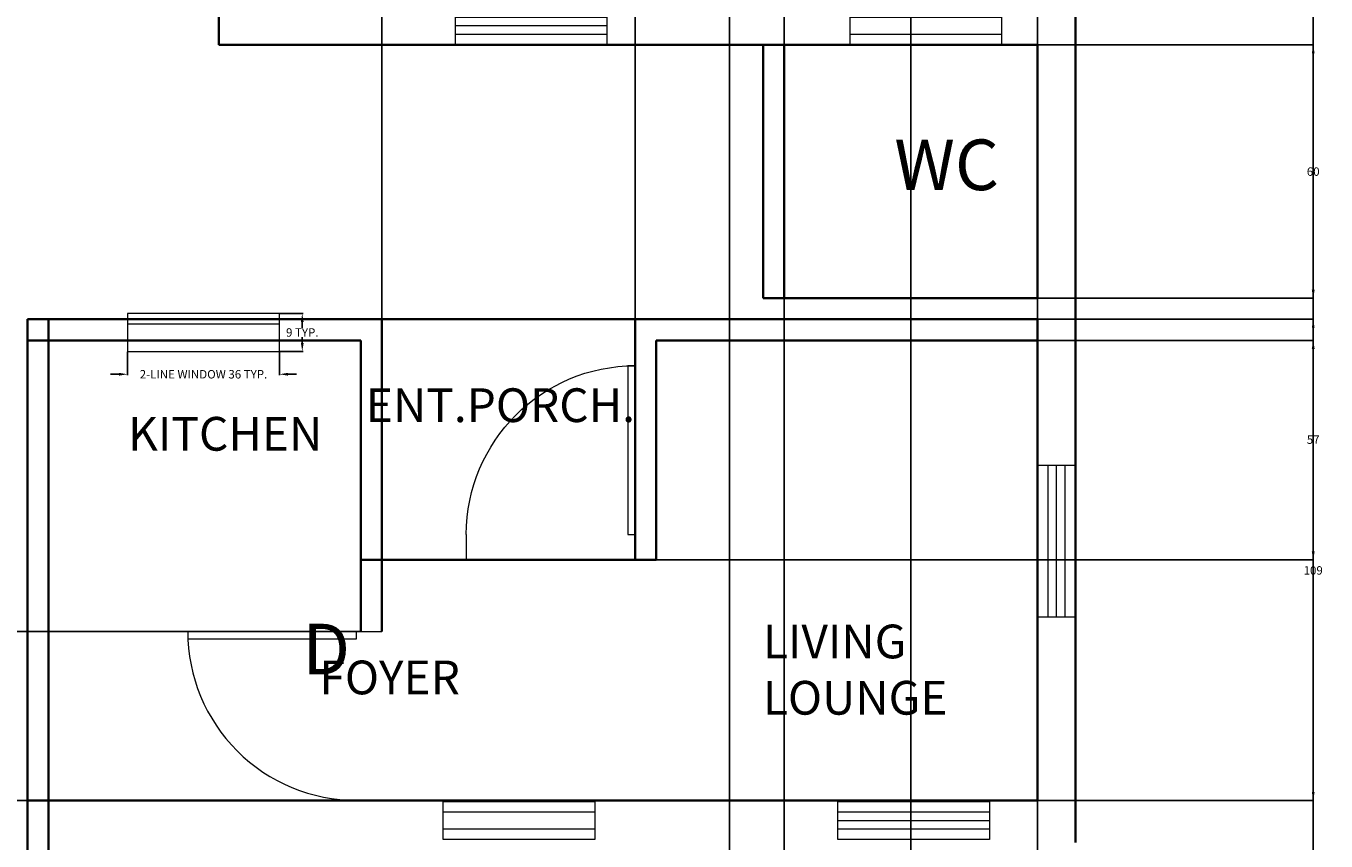
# Model space of a CAD drawing. Units: inches. Extents: x 190 to 836, y -241 to 999.
# Tile 4 of 9: x 528 to 836, y -8 to 185. Entities that reach past the tile are written whole.
import ezdxf

# ---------------------------------------------------------------- set-up
doc = ezdxf.new("R2010")
doc.units = ezdxf.units.IN
doc.header["$MEASUREMENT"] = 0
for name, color, linetype, lineweight in [('A-ANNO-DIMS', 2, 'Continuous', 18), ('A-ANNO-TEXT', 7, 'Continuous', 18), ('A-AREA-IDEN', 7, 'Continuous', 18), ('A-DOOR', 3, 'Continuous', 18), ('A-GLAZ', 4, 'Continuous', 18), ('A-WALL', 7, 'Continuous', 35)]:
    doc.layers.add(name, color=color, linetype=linetype, lineweight=lineweight)
doc.styles.get("Standard").update_dxf_attribs({"font": 'arial.ttf'})
doc.dimstyles.get("Standard").update_dxf_attribs({"dimtxt": 2, "dimasz": 2, "dimexe": 0.18, "dimexo": 0.0625, "dimgap": 0.09, "dimtad": 0, "dimtih": 1, "dimtoh": 1, "dimdec": 0, "dimzin": 0, "dimdsep": 46, "dimlunit": 3, "dimtxsty": 'Standard', "dimcen": 0.09, "dimadec": 0, "dimazin": 0, "dimtfac": 1, "dimtdec": 0, "dimtofl": 0, "dimtmove": 0, "dimatfit": 3, "dimfxl": 1, "dimtolj": 1, "dimtzin": 0, "dimarcsym": 0})

# ---------------------------------------------------------------- blocks, each defined once
blk = doc.blocks.new('*U2')
for p, q in [((0, 0), (0, 6)), ((40, 0), (40, 6))]:
    blk.add_line(p, q)
blk.add_lwpolyline([(0, 0), (0, -40), (1.75, -40), (1.75, 0)], close=True)
blk.add_arc((0, 0), 40, 270, 360)
blk = doc.blocks.new('*U5')
for p, q in [((0, 0), (0, -6)), ((40, 0), (40, -6))]:
    blk.add_line(p, q)
blk.add_lwpolyline([(0, 0), (0, 40), (1.75, 40), (1.75, 0)], close=True)
blk.add_arc((0, 0), 40, 0, 90)
blk = doc.blocks.new('WIN-36IN-9IN-3LINE')
for p, q in [((2.5, 36), (2.5, 0)), ((4.5, 36), (4.5, 0)), ((6.5, 36), (6.5, 0))]:
    blk.add_line(p, q)
blk.add_lwpolyline([(0, 0), (9, 0), (9, 36), (0, 36)], close=True)
blk = doc.blocks.new('WIN-36IN-9IN-2LINE')
for p, q in [((0, 6.5), (36, 6.5)), ((0, 2.5), (36, 2.5))]:
    blk.add_line(p, q)
blk.add_lwpolyline([(36, 0), (36, 9), (0, 9), (0, 0)], close=True)
blk = doc.blocks.new('*D12')
at = {"layer": 'A-ANNO-DIMS', "color": 0, "lineweight": -2, "transparency": 16777216}
for p, q in [((551.83, 107.85), (551.83, 102.33)), ((587.83, 107.85), (587.83, 102.33)), ((549.83, 102.51), (547.83, 102.51)), ((589.83, 102.51), (591.83, 102.51))]:
    blk.add_line(p, q, dxfattribs=at)
at = {"layer": 'A-ANNO-DIMS', "color": 0, "transparency": 16777216}
for points in [[(549.83, 102.84), (549.83, 102.18), (551.83, 102.51)], [(589.83, 102.84), (589.83, 102.18), (587.83, 102.51)]]:
    blk.add_solid(points, dxfattribs=at)
at = {"layer": 'Defpoints', "color": 0, "transparency": 16777216}
for p in [(551.83, 107.91), (587.83, 107.91), (551.83, 102.51)]:
    blk.add_point(p, dxfattribs=at)
at = {"layer": 'A-ANNO-DIMS', "color": 0, "transparency": 16777216, "insert": (569.83, 102.51), "char_height": 2, "attachment_point": 5}
blk.add_mtext('\\A1;2-LINE WINDOW 36 TYP.', dxfattribs=at)
blk = doc.blocks.new('*D13')
at = {"layer": 'A-ANNO-DIMS', "color": 0, "lineweight": -2, "transparency": 16777216}
for p, q in [((587.89, 116.91), (593.41, 116.91)), ((593.23, 114.91), (593.23, 113.52)), ((593.23, 109.91), (593.23, 111.3)), ((587.89, 107.91), (593.41, 107.91))]:
    blk.add_line(p, q, dxfattribs=at)
at = {"layer": 'A-ANNO-DIMS', "color": 0, "transparency": 16777216}
for points in [[(592.9, 114.91), (593.56, 114.91), (593.23, 116.91)], [(592.9, 109.91), (593.56, 109.91), (593.23, 107.91)]]:
    blk.add_solid(points, dxfattribs=at)
at = {"layer": 'Defpoints', "color": 0, "transparency": 16777216}
for p in [(587.83, 116.91), (587.83, 107.91), (593.23, 107.91)]:
    blk.add_point(p, dxfattribs=at)
at = {"layer": 'A-ANNO-DIMS', "color": 0, "transparency": 16777216, "insert": (593.23, 112.41), "char_height": 2, "attachment_point": 5}
blk.add_mtext('\\A1;9 TYP.', dxfattribs=at)
blk = doc.blocks.new('*D18')
at = {"layer": 'A-ANNO-DIMS', "color": 0, "lineweight": -2, "transparency": 16777216}
for p, q in [((776.5, 941.53), (832.94, 941.53)), ((832.76, 939.53), (832.76, 403.14)), ((832.76, -135.47), (832.76, 400.92)), ((776.5, -137.47), (832.94, -137.47))]:
    blk.add_line(p, q, dxfattribs=at)
at = {"layer": 'A-ANNO-DIMS', "color": 0, "transparency": 16777216}
for points in [[(832.43, 939.53), (833.1, 939.53), (832.76, 941.53)], [(832.43, -135.47), (833.1, -135.47), (832.76, -137.47)]]:
    blk.add_solid(points, dxfattribs=at)
at = {"layer": 'Defpoints', "color": 0, "transparency": 16777216}
for p in [(776.44, 941.53), (832.76, 941.53), (776.44, -137.47)]:
    blk.add_point(p, dxfattribs=at)
at = {"layer": 'A-ANNO-DIMS', "color": 0, "transparency": 16777216, "insert": (832.76, 402.03), "char_height": 2, "attachment_point": 5}
blk.add_mtext('\\A1;1079', dxfattribs=at)
blk = doc.blocks.new('*D31')
at = {"layer": 'A-ANNO-DIMS', "color": 0, "lineweight": -2, "transparency": 16777216}
for p, q in [((707.44, 855.47), (707.44, -239.95)), ((737.44, 855.47), (737.44, -239.95)), ((709.44, -239.77), (720.92, -239.77)), ((735.44, -239.77), (723.96, -239.77))]:
    blk.add_line(p, q, dxfattribs=at)
at = {"layer": 'A-ANNO-DIMS', "color": 0, "transparency": 16777216}
for points in [[(709.44, -239.44), (709.44, -240.11), (707.44, -239.77)], [(735.44, -239.44), (735.44, -240.11), (737.44, -239.77)]]:
    blk.add_solid(points, dxfattribs=at)
at = {"layer": 'Defpoints', "color": 0, "transparency": 16777216}
for p in [(707.44, 855.53), (737.44, 855.53), (707.44, -239.77)]:
    blk.add_point(p, dxfattribs=at)
at = {"layer": 'A-ANNO-DIMS', "color": 0, "transparency": 16777216, "insert": (722.44, -239.77), "char_height": 2, "attachment_point": 5}
blk.add_mtext('\\A1;30', dxfattribs=at)
blk = doc.blocks.new('*D41')
at = {"layer": 'A-ANNO-DIMS', "color": 0, "lineweight": -2, "transparency": 16777216}
for p, q in [((767.5, 110.53), (832.94, 110.53)), ((832.76, 108.53), (832.76, 57.14)), ((832.76, 3.53), (832.76, 54.92)), ((767.5, 1.53), (832.94, 1.53))]:
    blk.add_line(p, q, dxfattribs=at)
at = {"layer": 'A-ANNO-DIMS', "color": 0, "transparency": 16777216}
for points in [[(832.43, 108.53), (833.1, 108.53), (832.76, 110.53)], [(832.43, 3.53), (833.1, 3.53), (832.76, 1.53)]]:
    blk.add_solid(points, dxfattribs=at)
at = {"layer": 'Defpoints', "color": 0, "transparency": 16777216}
for p in [(767.44, 110.53), (832.76, 110.53), (767.44, 1.53)]:
    blk.add_point(p, dxfattribs=at)
at = {"layer": 'A-ANNO-DIMS', "color": 0, "transparency": 16777216, "insert": (832.76, 56.03), "char_height": 2, "attachment_point": 5}
blk.add_mtext('\\A1;109', dxfattribs=at)
blk = doc.blocks.new('*D42')
at = {"layer": 'A-ANNO-DIMS', "color": 0, "lineweight": -2, "transparency": 16777216}
for p, q in [((767.5, 180.53), (832.94, 180.53)), ((832.76, 178.53), (832.76, 151.64)), ((832.76, 122.53), (832.76, 149.42)), ((767.5, 120.53), (832.94, 120.53))]:
    blk.add_line(p, q, dxfattribs=at)
at = {"layer": 'A-ANNO-DIMS', "color": 0, "transparency": 16777216}
for points in [[(832.43, 178.53), (833.1, 178.53), (832.76, 180.53)], [(832.43, 122.53), (833.1, 122.53), (832.76, 120.53)]]:
    blk.add_solid(points, dxfattribs=at)
at = {"layer": 'Defpoints', "color": 0, "transparency": 16777216}
for p in [(767.44, 180.53), (832.76, 180.53), (767.44, 120.53)]:
    blk.add_point(p, dxfattribs=at)
at = {"layer": 'A-ANNO-DIMS', "color": 0, "transparency": 16777216, "insert": (832.76, 150.53), "char_height": 2, "attachment_point": 5}
blk.add_mtext('\\A1;60', dxfattribs=at)
blk = doc.blocks.new('*D43')
at = {"layer": 'A-ANNO-DIMS', "color": 0, "lineweight": -2, "transparency": 16777216}
for p, q in [((694.44, -128.41), (694.44, 998.02)), ((767.44, -128.41), (767.44, 998.02)), ((696.44, 997.84), (729.43, 997.84)), ((765.44, 997.84), (732.45, 997.84))]:
    blk.add_line(p, q, dxfattribs=at)
at = {"layer": 'A-ANNO-DIMS', "color": 0, "transparency": 16777216}
for points in [[(696.44, 998.17), (696.44, 997.5), (694.44, 997.84)], [(765.44, 998.17), (765.44, 997.5), (767.44, 997.84)]]:
    blk.add_solid(points, dxfattribs=at)
at = {"layer": 'Defpoints', "color": 0, "transparency": 16777216}
for p in [(767.44, 997.84), (694.44, -128.47), (767.44, -128.47)]:
    blk.add_point(p, dxfattribs=at)
at = {"layer": 'A-ANNO-DIMS', "color": 0, "transparency": 16777216, "insert": (730.94, 997.84), "char_height": 2, "attachment_point": 5}
blk.add_mtext('\\A1;73', dxfattribs=at)
blk = doc.blocks.new('*D45')
at = {"layer": 'A-ANNO-DIMS', "color": 0, "lineweight": -2, "transparency": 16777216}
for p, q in [((612.1, 115.59), (612.1, 998.02)), ((672.1, 115.59), (672.1, 998.02)), ((614.1, 997.84), (640.58, 997.84)), ((670.1, 997.84), (643.62, 997.84))]:
    blk.add_line(p, q, dxfattribs=at)
at = {"layer": 'A-ANNO-DIMS', "color": 0, "transparency": 16777216}
for points in [[(614.1, 998.17), (614.1, 997.5), (612.1, 997.84)], [(670.1, 998.17), (670.1, 997.5), (672.1, 997.84)]]:
    blk.add_solid(points, dxfattribs=at)
at = {"layer": 'Defpoints', "color": 0, "transparency": 16777216}
for p in [(672.1, 997.84), (612.1, 115.53), (672.1, 115.53)]:
    blk.add_point(p, dxfattribs=at)
at = {"layer": 'A-ANNO-DIMS', "color": 0, "transparency": 16777216, "insert": (642.1, 997.84), "char_height": 2, "attachment_point": 5}
blk.add_mtext('\\A1;60', dxfattribs=at)
blk = doc.blocks.new('*D46')
at = {"layer": 'A-ANNO-DIMS', "color": 0, "lineweight": -2, "transparency": 16777216}
for p, q in [((707.44, 120.59), (707.44, 998.02)), ((767.44, 120.59), (767.44, 998.02)), ((709.44, 997.84), (735.92, 997.84)), ((765.44, 997.84), (738.97, 997.84))]:
    blk.add_line(p, q, dxfattribs=at)
at = {"layer": 'A-ANNO-DIMS', "color": 0, "transparency": 16777216}
for points in [[(709.44, 998.17), (709.44, 997.5), (707.44, 997.84)], [(765.44, 998.17), (765.44, 997.5), (767.44, 997.84)]]:
    blk.add_solid(points, dxfattribs=at)
at = {"layer": 'Defpoints', "color": 0, "transparency": 16777216}
for p in [(767.44, 997.84), (707.44, 120.53), (767.44, 120.53)]:
    blk.add_point(p, dxfattribs=at)
at = {"layer": 'A-ANNO-DIMS', "color": 0, "transparency": 16777216, "insert": (737.44, 997.84), "char_height": 2, "attachment_point": 5}
blk.add_mtext('\\A1;60', dxfattribs=at)
blk = doc.blocks.new('*D47')
at = {"layer": 'A-ANNO-DIMS', "color": 0, "lineweight": -2, "transparency": 16777216}
for p, q in [((612.16, 115.53), (832.94, 115.53)), ((832.76, 113.53), (832.76, 88.14)), ((832.76, 60.53), (832.76, 85.92)), ((607.16, 58.53), (832.94, 58.53))]:
    blk.add_line(p, q, dxfattribs=at)
at = {"layer": 'A-ANNO-DIMS', "color": 0, "transparency": 16777216}
for points in [[(832.43, 113.53), (833.1, 113.53), (832.76, 115.53)], [(832.43, 60.53), (833.1, 60.53), (832.76, 58.53)]]:
    blk.add_solid(points, dxfattribs=at)
at = {"layer": 'Defpoints', "color": 0, "transparency": 16777216}
for p in [(612.1, 115.53), (832.76, 115.53), (607.1, 58.53)]:
    blk.add_point(p, dxfattribs=at)
at = {"layer": 'A-ANNO-DIMS', "color": 0, "transparency": 16777216, "insert": (832.76, 87.03), "char_height": 2, "attachment_point": 5}
blk.add_mtext('\\A1;57', dxfattribs=at)
blk = doc.blocks.new('*D49')
at = {"layer": 'A-ANNO-DIMS', "color": 0, "lineweight": -2, "transparency": 16777216}
for p, q in [((607.04, 41.53), (193.96, 41.53)), ((194.14, 39.53), (194.14, 22.64)), ((194.14, 3.53), (194.14, 20.42)), ((606.04, 1.53), (193.96, 1.53))]:
    blk.add_line(p, q, dxfattribs=at)
at = {"layer": 'A-ANNO-DIMS', "color": 0, "transparency": 16777216}
for points in [[(193.8, 39.53), (194.47, 39.53), (194.14, 41.53)], [(193.8, 3.53), (194.47, 3.53), (194.14, 1.53)]]:
    blk.add_solid(points, dxfattribs=at)
at = {"layer": 'Defpoints', "color": 0, "transparency": 16777216}
for p in [(607.1, 41.53), (194.14, 1.53), (606.1, 1.53)]:
    blk.add_point(p, dxfattribs=at)
at = {"layer": 'A-ANNO-DIMS', "color": 0, "transparency": 16777216, "insert": (194.14, 21.53), "char_height": 2, "attachment_point": 5}
blk.add_mtext('\\A1;40', dxfattribs=at)

msp = doc.modelspace()

# ---------------------------------------------------------------- linework, layer by layer
at = {"layer": 'A-WALL'}
for p, q in [((776.4421, -8.4687), (776.4421, 565.5313)), ((573.4421, 342.5313), (573.4421, 180.5313)), ((573.4421, 180.5313), (767.4421, 180.5313)), ((702.4421, 120.5313), (702.4421, 180.5313)), ((707.4421, 120.5313), (707.4421, 180.5313)), ((767.4421, 120.5313), (767.4421, 180.5313)), ((702.4421, 120.5313), (767.4421, 120.5313)), ((767.4421, 115.5313), (528.0998, 115.5313)), ((528.0998, 115.5313), (528.0998, -128.4687)), ((533.0998, 115.5313), (533.0998, -128.4687)), ((573.4421, 115.5313), (767.4421, 115.5313)), ((612.0998, 115.5313), (612.0998, 41.5313)), ((672.0998, 115.5313), (672.0998, 58.5313)), ((767.4421, 1.5313), (767.4421, 115.5313)), ((767.4421, 1.5313), (767.4421, 115.5313)), ((607.0998, 110.5313), (528.0998, 110.5313)), ((607.0998, 110.5313), (607.0998, 41.5313)), ((767.4421, 110.5313), (677.0998, 110.5313)), ((677.0998, 110.5313), (677.0998, 58.5313)), ((607.0998, 58.5313), (677.0998, 58.5313)), ((528.0998, 1.5313), (767.4421, 1.5313))]:
    msp.add_line(p, q, dxfattribs=at)

# ---------------------------------------------------------------- block references
at = {"layer": 'A-DOOR', "xscale": -1, "rotation": 360}
msp.add_blockref('*U5', (672.0998, 64.5313), dxfattribs=at)
at = {"layer": 'A-DOOR', "rotation": 269.9999999999999}
msp.add_blockref('*U2', (606.0998, 41.5313), dxfattribs=at)
at = {"layer": 'A-GLAZ'}
for name, p, rotation in [('WIN-36IN-9IN-3LINE', (629.4485, 189.5315), 269.9999999999995), ('WIN-36IN-9IN-2LINE', (758.9673, 189.5317), 180), ('WIN-36IN-9IN-2LINE', (587.8309, 116.9119), 180)]:
    msp.add_blockref(name, p, dxfattribs=dict(at, rotation=rotation))
at = {"layer": 'A-GLAZ', "extrusion": (0, 0, -1), "zscale": -1}
for name, p, rotation in [('WIN-36IN-9IN-3LINE', (-767.4582, 80.9814), 180), ('WIN-36IN-9IN-2LINE', (-626.579, 1.3014), 180), ('WIN-36IN-9IN-3LINE', (-756.0978, 1.3012), 269.9999999999996)]:
    msp.add_blockref(name, p, dxfattribs=dict(at, rotation=rotation))

# ---------------------------------------------------------------- texts
at = {"layer": 'A-ANNO-TEXT', "insert": (604.5511, 43.4036), "char_height": 12, "attachment_point": 3}
msp.add_mtext_dynamic_manual_height_columns('D', width=8.765037, gutter_width=1, heights=[0], dxfattribs=at)
at = {"layer": 'A-AREA-IDEN'}
for s, width, insert, char_height, attachment_point in [('WC', 21.816424, (733.4972, 158.137), 12, 1), ('ENT.PORCH.', 33.040256, (608.2937, 91.1796), 8, 7), ('KITCHEN', 33.040256, (551.9708, 84.4054), 8, 7), ('LIVING LOUNGE ', 33.040256, (702.3714, 21.8555), 8, 7), ('FOYER', 33.040256, (597.3069, 26.6704), 8, 7)]:
    msp.add_mtext_dynamic_manual_height_columns(s, width=width, gutter_width=1, heights=[0], dxfattribs=dict(at, insert=insert, char_height=char_height, attachment_point=attachment_point))

# ---------------------------------------------------------------- dimensions: what is measured, and where the dimension line sits
at = {"layer": 'A-ANNO-DIMS'}
for base, p1, p2, picture, middle in [((672.0998, 997.8363), (612.0998, 115.5313), (672.0998, 115.5313), '*D45', (642.0998, 997.8363)), ((767.4421, 997.8363), (694.4376, -128.4687), (767.4421, -128.4687), '*D43', (730.9399, 997.8363)), ((767.4421, 997.8363), (707.4421, 120.5313), (767.4421, 120.5313), '*D46', (737.4421, 997.8363)), ((707.4421, -239.7737), (737.4421, 855.5313), (707.4421, 855.5313), '*D31', (722.4421, -239.7737))]:
    dim = msp.add_linear_dim(base=base, p1=p1, p2=p2, dimstyle='Standard', override={"dimdec": 0, "dimlfac": 1, "dimrnd": 0, "dimzin": 0, "dimdsep": 46, "dimlunit": 2}, dxfattribs=at)
    dim.commit()
    dim.dimension.update_dxf_attribs({"geometry": picture, "text_midpoint": middle})
for base, p1, p2, picture, middle in [((832.7634, 941.5313), (776.4421, -137.4687), (776.4421, 941.5313), '*D18', (832.7634, 402.0313)), ((832.7634, 180.5313), (767.4421, 120.5313), (767.4421, 180.5313), '*D42', (832.7634, 150.5313)), ((832.7634, 115.5313), (607.0998, 58.5313), (612.0998, 115.5313), '*D47', (832.7634, 87.0313)), ((832.7634, 110.5313), (767.4421, 1.5313), (767.4421, 110.5313), '*D41', (832.7634, 56.0313)), ((194.1371, 1.5313), (607.0998, 41.5313), (606.0998, 1.5313), '*D49', (194.1371, 21.5313))]:
    dim = msp.add_linear_dim(base=base, p1=p1, p2=p2, angle=90, dimstyle='Standard', override={"dimdec": 0, "dimlfac": 1, "dimrnd": 0, "dimzin": 0, "dimdsep": 46, "dimlunit": 2}, dxfattribs=at)
    dim.commit()
    dim.dimension.update_dxf_attribs({"geometry": picture, "text_midpoint": middle})
for base, p1, p2, angle, text, picture, middle in [((593.2304, 107.9116), (587.8304, 116.9116), (587.8304, 107.9116), 270, '<> TYP.', '*D13', (593.2304, 112.4116)), ((551.8304, 102.5116), (587.8304, 107.9116), (551.8304, 107.9116), 180, '2-LINE WINDOW <> TYP.', '*D12', (569.8304, 102.5116))]:
    dim = msp.add_linear_dim(base=base, p1=p1, p2=p2, angle=angle, text=text, dimstyle='Standard', override={"dimdec": 0, "dimlfac": 1, "dimrnd": 0, "dimzin": 0, "dimdsep": 46, "dimlunit": 2}, dxfattribs=at)
    dim.commit()
    dim.dimension.update_dxf_attribs({"geometry": picture, "text_midpoint": middle})

doc.saveas('drawing.dxf')
